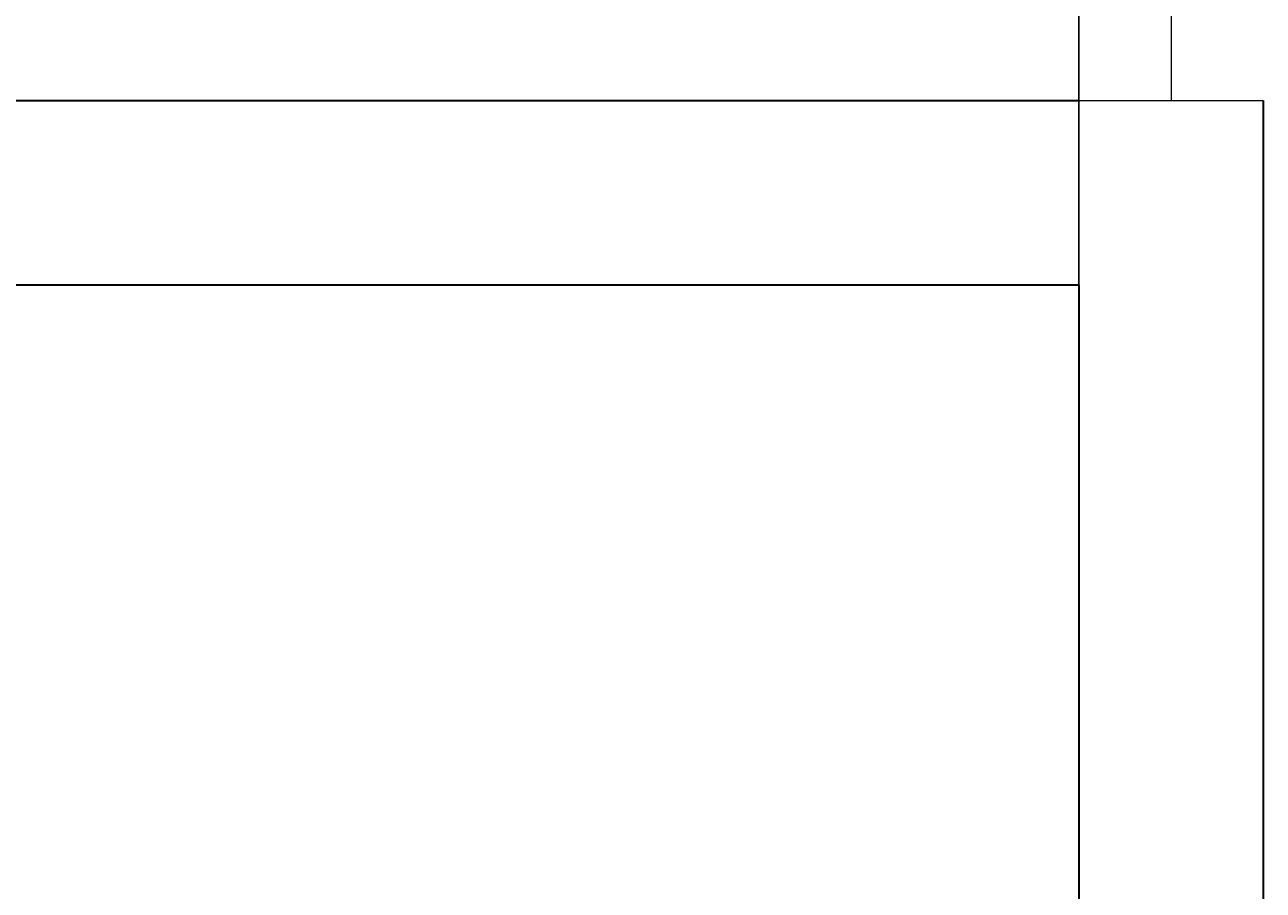
# Model space of a CAD drawing. Units: inches. Extents: x 1088 to 1703, y 668 to 1875.
# Tile 38 of 45: x 1560 to 1590, y 1654 to 1675. Entities that reach past the tile are written whole.
import ezdxf

# ---------------------------------------------------------------- set-up
doc = ezdxf.new("R2010")
doc.units = ezdxf.units.IN
for name, color, linetype, lineweight in [('A-ANNO-DIMS', 2, 'Continuous', 18), ('A-DOOR', 4, 'Continuous', 18), ('A-WALL', 7, 'Continuous', 35)]:
    doc.layers.add(name, color=color, linetype=linetype, lineweight=lineweight)
doc.styles.get("Standard").update_dxf_attribs({"font": 'arial.ttf'})
doc.dimstyles.get("Standard").update_dxf_attribs({"dimtxt": 0.18, "dimasz": 0.18, "dimexe": 0.18, "dimexo": 0.0625, "dimgap": 0.09, "dimtad": 0, "dimtih": 1, "dimtoh": 1, "dimdec": 4, "dimzin": 0, "dimdsep": 46, "dimtxsty": 'Standard', "dimcen": 0.09, "dimadec": 0, "dimazin": 0, "dimtfac": 1, "dimtdec": 4, "dimtofl": 0, "dimtmove": 0, "dimatfit": 3, "dimfxl": 1, "dimtolj": 1, "dimtzin": 0, "dimarcsym": 0})

# ---------------------------------------------------------------- blocks, each defined once
blk = doc.blocks.new('*D32')
at = {"layer": 'A-ANNO-DIMS', "color": 0, "lineweight": -2, "transparency": 16777216}
for p, q in [((1550.595, 1373.121), (1550.595, 1857.788)), ((1550.775, 1857.608), (1567.825, 1857.608)), ((1585.665, 1857.608), (1568.614, 1857.608)), ((1585.845, 1360.983), (1585.845, 1857.788))]:
    blk.add_line(p, q, dxfattribs=at)
at = {"layer": 'A-ANNO-DIMS', "color": 0, "transparency": 16777216}
for points in [[(1550.775, 1857.638), (1550.775, 1857.578), (1550.595, 1857.608)], [(1585.665, 1857.638), (1585.665, 1857.578), (1585.845, 1857.608)]]:
    blk.add_solid(points, dxfattribs=at)
at = {"layer": 'Defpoints', "color": 0, "transparency": 16777216}
for p in [(1585.845, 1857.608), (1550.595, 1373.058), (1585.845, 1360.921)]:
    blk.add_point(p, dxfattribs=at)
at = {"layer": 'A-ANNO-DIMS', "color": 0, "transparency": 16777216, "insert": (1568.22, 1857.608), "char_height": 0.18, "attachment_point": 5}
blk.add_mtext('\\A1;35.25', dxfattribs=at)

msp = doc.modelspace()

# ---------------------------------------------------------------- linework, layer by layer
at = {"layer": 'A-DOOR'}
for p, q in [((1588.095, 1736.337), (1588.095, 1673.058)), ((1585.845, 1673.058), (1590.345, 1673.058))]:
    msp.add_line(p, q, dxfattribs=at)
at = {"layer": 'A-WALL'}
for p, q in [((1481.681, 1673.058), (1585.845, 1673.058)), ((1590.345, 1673.058), (1590.345, 1539.558)), ((1489.845, 1668.558), (1585.845, 1668.558)), ((1585.845, 1668.558), (1585.845, 1544.058)), ((1585.845, 1668.558), (1585.845, 1608.558))]:
    msp.add_line(p, q, dxfattribs=at)

# ---------------------------------------------------------------- dimensions: what is measured, and where the dimension line sits
at = {"layer": 'A-ANNO-DIMS'}
dim = msp.add_linear_dim(base=(1585.845, 1857.608), p1=(1550.595, 1373.058), p2=(1585.845, 1360.921), dimstyle='Standard', override={"dimdec": 2, "dimlfac": 1, "dimrnd": 0, "dimzin": 0, "dimdsep": 46, "dimlunit": 2}, dxfattribs=at)
dim.commit()
dim.dimension.update_dxf_attribs({"geometry": '*D32', "text_midpoint": (1568.22, 1857.608)})

doc.saveas('drawing.dxf')
